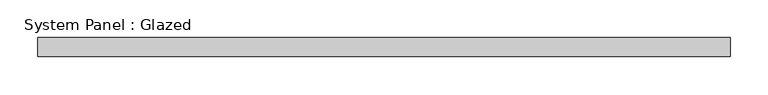
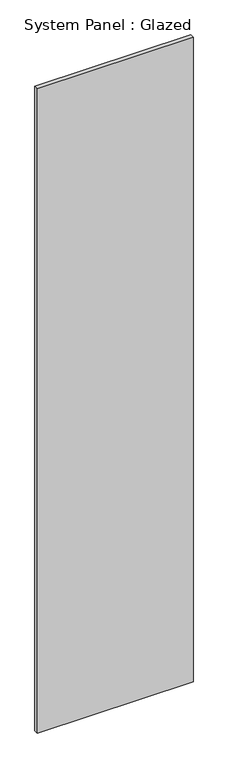
"""IFC4 building model written with IfcOpenShell, lengths in millimetres: plate geometry, System Panel : Glazed."""

from ifc_helpers import new_model, si_unit, origin, origin_with_axes, place, context, project, spatial, polyline, outline, extrude, source, transform, mapped, element, save


def system_panel_glazed_234dce3e(model_context):
    return source(origin(), model_context, "Body", "SweptSolid", [
        extrude(outline(polyline([(457.2, 24.5), (-457.2, 24.5), (-457.2, 49.5), (457.2, 49.5), (457.2, 24.5)])), origin_with_axes(), (0.0, 0.0, 1.0), 4000.0),
    ])


if __name__ == "__main__":
    model = new_model("IFC4")
    model_context = context("Model", 3, world=origin())
    ifc_project = project(units=[si_unit("LENGTHUNIT", "METRE", prefix="MILLI")], contexts=[model_context])
    site = spatial("IfcSite", under=ifc_project)
    building = spatial("IfcBuilding", under=site)
    placement = place(None, origin())
    system_panel_glazed_shape = system_panel_glazed_234dce3e(model_context)
    element("IfcPlate", 1, ObjectType="System Panel : Glazed", at=placement, inside=building, context=model_context, shape_type="MappedRepresentation", body=[
        mapped(system_panel_glazed_shape, transform((0.0, 0.0, 0.0), x_axis=(1.0, 0.0, 0.0), y_axis=(0.0, 1.0, 0.0), z_axis=(0.0, 0.0, 1.0))),
    ])
    save(model, "model.ifc")

# Revit data of these elements
# Type "System Panel : Glazed"
#   Keynote = "H11"
#   Construction Type Id = "GSP4R"
#   Analytic Construction = "1/8 in Pilkington single glazing"
#   Visual Light Transmittance = 0.9
#   Solar Heat Gain Coefficient = 0.86
#   Heat Transfer Coefficient (U) = 6.7069 W/(m²·K)
#   Define Thermal Properties by = 1
# Element 1 (IfcPlate, "System Panel : Glazed")
#   Materials on its faces: "Glass"
# Materials
#   "Glass": class "Glass", colour RGB 0 128 192, transparency 0.9, Description = "Soda Lime Glass", Cost = 0
